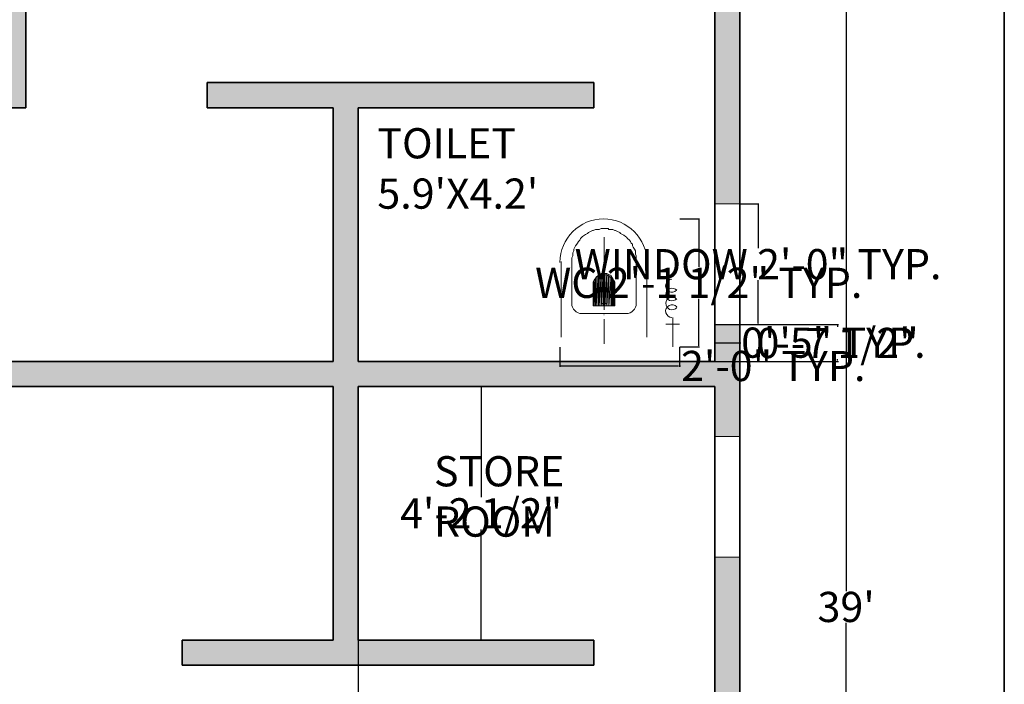
# Model space of a CAD drawing. Units: inches. Extents: x 717 to 1167, y 2046 to 2594.
# Tile 5 of 6: x 972 to 1167, y 2298 to 2430. Entities that reach past the tile are written whole.
import ezdxf

# ---------------------------------------------------------------- set-up
doc = ezdxf.new("R2010")
doc.units = ezdxf.units.IN
doc.header["$MEASUREMENT"] = 0
for name, color, linetype, lineweight in [('A-ANNO-DIMS', 2, 'Continuous', 18), ('A-ANNO-TTLB', 7, 'Continuous', 35), ('A-AREA-IDEN', 7, 'Continuous', 18), ('A-FLOR-FIXT', 8, 'Continuous', 18), ('A-GLAZ', 4, 'Continuous', 18), ('A-WALL', 7, 'Continuous', 35), ('A-WALL-PATT', 140, 'Continuous', 13)]:
    doc.layers.add(name, color=color, linetype=linetype, lineweight=lineweight)
doc.styles.get("Standard").update_dxf_attribs({"font": 'arial.ttf'})
doc.dimstyles.get("Standard").update_dxf_attribs({"dimtxt": 6, "dimasz": 0.18, "dimexe": 0.18, "dimexo": 0.0625, "dimgap": 0.09, "dimtad": 0, "dimtih": 1, "dimtoh": 1, "dimdec": 1, "dimzin": 0, "dimdsep": 46, "dimlunit": 3, "dimtxsty": 'Standard', "dimcen": 0.09, "dimadec": 0, "dimazin": 0, "dimtfac": 1, "dimtdec": 1, "dimtofl": 0, "dimtmove": 0, "dimatfit": 3, "dimfxl": 1, "dimtolj": 1, "dimtzin": 0, "dimarcsym": 0})

# ---------------------------------------------------------------- blocks, each defined once
blk = doc.blocks.new('*D5')
at = {"layer": 'A-ANNO-DIMS', "color": 0, "lineweight": -2, "transparency": 16777216}
for p, q in [((1114.78, 2547.57), (1135.98, 2547.57)), ((1135.8, 2547.39), (1135.8, 2316.73)), ((1135.8, 2079.75), (1135.8, 2310.41)), ((1114.78, 2079.57), (1135.98, 2079.57))]:
    blk.add_line(p, q, dxfattribs=at)
at = {"layer": 'A-ANNO-DIMS', "color": 0, "transparency": 16777216}
for points in [[(1135.77, 2547.39), (1135.83, 2547.39), (1135.8, 2547.57)], [(1135.77, 2079.75), (1135.83, 2079.75), (1135.8, 2079.57)]]:
    blk.add_solid(points, dxfattribs=at)
at = {"layer": 'Defpoints', "color": 0, "transparency": 16777216}
for p in [(1114.71, 2547.57), (1114.71, 2079.57), (1135.8, 2079.57)]:
    blk.add_point(p, dxfattribs=at)
at = {"layer": 'A-ANNO-DIMS', "color": 0, "transparency": 16777216, "insert": (1135.8, 2313.57), "char_height": 6, "attachment_point": 5}
blk.add_mtext("\\A1;39'", dxfattribs=at)
blk = doc.blocks.new('WC-PLAN')
h = blk.add_hatch(color=256)
h.paths.add_polyline_path([(7.21, 8.12), (7.21, 13.81), (7.05, 8.12)])
h.paths.add_polyline_path([(7.21, 13.81), (7.05, 8.12), (7.05, 13.58)])
h = blk.add_hatch(color=256)
h.paths.add_polyline_path([(7.59, 8.12), (7.59, 14.19), (7.21, 8.12)])
h.paths.add_polyline_path([(7.59, 14.19), (7.21, 8.12), (7.21, 13.81)])
h = blk.add_hatch(color=256)
h.paths.add_polyline_path([(7.81, 8.12), (7.81, 14.34), (7.59, 8.12)])
h.paths.add_polyline_path([(7.81, 14.34), (7.59, 8.12), (7.59, 14.19)])
h = blk.add_hatch(color=256)
h.paths.add_polyline_path([(8.19, 8.12), (8.19, 14.56), (7.81, 8.12)])
h.paths.add_polyline_path([(8.19, 14.56), (7.81, 8.12), (7.81, 14.34)])
h = blk.add_hatch(color=256)
h.paths.add_polyline_path([(8.57, 8.12), (8.57, 14.56), (8.19, 8.12)])
h.paths.add_polyline_path([(8.57, 14.56), (8.19, 8.12), (8.19, 14.56)])
h = blk.add_hatch(color=256)
h.paths.add_polyline_path([(8.95, 8.12), (8.95, 14.56), (8.57, 8.12)])
h.paths.add_polyline_path([(8.95, 14.56), (8.57, 8.12), (8.57, 14.56)])
h = blk.add_hatch(color=256)
h.paths.add_polyline_path([(9.33, 8.12), (9.33, 14.56), (8.95, 8.12)])
h.paths.add_polyline_path([(9.33, 14.56), (8.95, 8.12), (8.95, 14.56)])
h = blk.add_hatch(color=256)
h.paths.add_polyline_path([(9.71, 8.12), (9.71, 14.34), (9.33, 8.12)])
h.paths.add_polyline_path([(9.71, 14.34), (9.33, 8.12), (9.33, 14.56)])
h = blk.add_hatch(color=256)
h.paths.add_polyline_path([(10.16, 8.12), (10.16, 14.19), (9.71, 8.12)])
h.paths.add_polyline_path([(10.16, 14.19), (9.71, 8.12), (9.71, 14.34)])
h = blk.add_hatch(color=256)
h.paths.add_polyline_path([(10.32, 8.12), (10.32, 13.81), (10.16, 8.12)])
h.paths.add_polyline_path([(10.32, 13.81), (10.16, 8.12), (10.16, 14.19)])
h = blk.add_hatch(color=256)
h.paths.add_polyline_path([(10.54, 8.12), (10.54, 13.58), (10.32, 8.12)])
h.paths.add_polyline_path([(10.54, 13.58), (10.32, 8.12), (10.32, 13.81)])
h = blk.add_hatch(color=256)
h.paths.add_polyline_path([(6.83, 8.12), (6.83, 13.2), (6.6, 8.12)])
h.paths.add_polyline_path([(6.83, 13.2), (6.6, 8.12), (6.6, 12.82)])
h.paths.add_polyline_path([(6.6, 8.12), (6.6, 12.82), (6.6, 12.44)])
h = blk.add_hatch(color=256)
h.paths.add_polyline_path([(7.05, 8.12), (7.05, 13.58), (6.83, 8.12)])
h.paths.add_polyline_path([(7.05, 13.58), (6.83, 8.12), (6.83, 13.2)])
h = blk.add_hatch(color=256)
h.paths.add_polyline_path([(10.7, 8.12), (10.7, 13.2), (10.54, 8.12)])
h.paths.add_polyline_path([(10.7, 13.2), (10.54, 8.12), (10.54, 13.58)])
h = blk.add_hatch(color=256)
h.paths.add_polyline_path([(10.92, 8.12), (10.92, 12.82), (10.7, 8.12)])
h.paths.add_polyline_path([(10.92, 12.82), (10.7, 8.12), (10.7, 13.2)])
for points in [[(2.35, 15.93), (2.35, 16.69), (2.35, 17.3), (2.35, 17.67), (2.58, 18.05), (2.58, 18.43), (2.58, 18.66), (2.73, 19.04), (2.73, 19.42), (2.96, 19.8), (3.11, 20.03), (3.34, 20.41), (3.49, 20.56), (3.72, 20.94), (3.94, 21.16), (4.1, 21.54), (4.32, 21.77), (4.48, 21.92), (4.85, 22.15), (5.08, 22.3), (5.46, 22.53), (5.69, 22.68), (6.07, 22.91), (6.45, 23.14), (6.6, 23.14), (7.05, 23.29), (7.43, 23.29), (7.81, 23.29), (8.19, 23.52), (8.8, 23.52), (9.56, 23.52), (9.71, 23.29), (10.16, 23.29), (10.54, 23.29), (10.92, 23.14), (11.07, 23.14), (11.45, 22.91), (11.91, 22.68), (12.06, 22.53), (12.44, 22.3), (12.67, 22.15), (13.05, 21.92), (13.2, 21.77), (13.43, 21.54), (13.81, 21.16), (14.03, 20.94), (14.18, 20.56), (14.41, 20.41), (14.41, 20.03), (14.56, 19.8), (14.79, 19.42), (15.02, 19.04), (15.02, 18.66), (15.02, 18.43), (15.17, 18.05), (15.17, 17.67), (15.17, 17.3), (15.17, 16.69), (15.17, 15.93)], [(8.8, 16.92), (8.8, 21.77), (8.8, 21.77)], [(0.23, 1.9), (0.23, 16.92), (0.23, 16.92)], [(2.35, 8.72), (2.35, 15.93), (2.35, 15.93)], [(15.17, 8.72), (15.17, 15.93), (15.17, 15.93)], [(17.29, 1.9), (17.29, 16.92), (17.29, 16.92)], [(8.8, 7.36), (8.8, 14.94), (8.8, 14.94)], [(6.6, 8.12), (6.6, 12.44), (6.6, 12.44)], [(10.92, 8.12), (10.92, 12.44), (10.92, 12.44)], [(6.6, 8.12), (10.92, 8.12), (10.92, 8.12)], [(8.34, 8.57), (8.57, 8.57), (8.8, 8.57)], [(8.34, 8.57), (8.34, 8.5), (8.34, 8.5)], [(8.8, 8.57), (8.72, 8.5), (8.72, 8.5)], [(8.8, 8.57), (8.95, 8.57), (9.18, 8.57)], [(9.18, 8.57), (9.18, 8.5), (9.18, 8.5)], [(4.48, 6.6), (13.2, 6.6), (13.2, 6.6)], [(8.8, 6.37), (8.72, 6.37), (8.72, 6.37)], [(8.8, 0.61), (8.8, 5.46), (8.8, 5.46)], [(21.03, 4.48), (23.77, 4.48), (23.77, 4.48)], [(22.4, 0), (22.4, 5.84), (22.4, 5.84)]]:
    blk.add_lwpolyline(points)
for points in [[(7.21, 8.12), (7.21, 13.81), (7.05, 8.12)], [(7.21, 13.81), (7.05, 8.12), (7.05, 13.58)], [(7.59, 8.12), (7.59, 14.19), (7.21, 8.12)], [(7.59, 14.19), (7.21, 8.12), (7.21, 13.81)], [(7.81, 8.12), (7.81, 14.34), (7.59, 8.12)], [(7.81, 14.34), (7.59, 8.12), (7.59, 14.19)], [(8.19, 8.12), (8.19, 14.56), (7.81, 8.12)], [(8.19, 14.56), (7.81, 8.12), (7.81, 14.34)], [(8.57, 8.12), (8.57, 14.56), (8.19, 8.12)], [(8.57, 14.56), (8.19, 8.12), (8.19, 14.56)], [(8.95, 8.12), (8.95, 14.56), (8.57, 8.12)], [(8.95, 14.56), (8.57, 8.12), (8.57, 14.56)], [(9.33, 8.12), (9.33, 14.56), (8.95, 8.12)], [(9.33, 14.56), (8.95, 8.12), (8.95, 14.56)], [(9.71, 14.34), (9.33, 8.12), (9.33, 14.56)], [(9.71, 8.12), (9.71, 14.34), (9.33, 8.12)], [(10.16, 14.19), (9.71, 8.12), (9.71, 14.34)], [(10.16, 8.12), (10.16, 14.19), (9.71, 8.12)], [(10.32, 13.81), (10.16, 8.12), (10.16, 14.19)], [(10.32, 8.12), (10.32, 13.81), (10.16, 8.12)], [(10.54, 13.58), (10.32, 8.12), (10.32, 13.81)], [(6.83, 8.12), (6.83, 13.2), (6.6, 8.12)], [(6.83, 13.2), (6.6, 8.12), (6.6, 12.82)], [(6.6, 8.12), (6.6, 12.82), (6.6, 12.44)], [(6.6, 12.82), (6.6, 8.12), (6.6, 8.12)], [(7.05, 8.12), (7.05, 13.58), (6.83, 8.12)], [(7.05, 13.58), (6.83, 8.12), (6.83, 13.2)], [(10.54, 8.12), (10.54, 13.58), (10.32, 8.12)], [(10.7, 13.2), (10.54, 8.12), (10.54, 13.58)], [(10.7, 8.12), (10.7, 13.2), (10.54, 8.12)], [(10.92, 12.82), (10.7, 8.12), (10.7, 13.2)], [(10.92, 8.12), (10.92, 12.82), (10.7, 8.12)], [(10.92, 12.44), (10.92, 8.12), (10.92, 12.82)], [(10.92, 8.12), (10.92, 12.44)]]:
    blk.add_lwpolyline(points, close=True)
for points, knots in [([(17.29, 16.76), (17.29, 21.54), (13.43, 25.41), (8.65, 25.41), (8.65, 25.41), (3.87, 25.41), (0, 21.54), (0, 16.76)], [0, 0, 0, 0, 0.125, 0.125, 0.125, 0.125001, 1, 1, 1, 1]), ([(10.7, 12.29), (10.7, 13.43), (9.79, 14.34), (8.65, 14.34), (8.65, 14.34), (7.51, 14.34), (6.6, 13.43), (6.6, 12.29)], [0, 0, 0, 0, 0.125, 0.125, 0.125, 0.125001, 1, 1, 1, 1]), ([(22.25, 13.43), (21.72, 13.43), (21.19, 12.97), (21.03, 12.44), (21.03, 12.44), (20.88, 11.91), (21.19, 11.3), (21.64, 11), (21.64, 11), (22.17, 10.77), (22.78, 10.85), (23.16, 11.23)], [0, 0, 0, 0, 0.083333, 0.083333, 0.083333, 0.083334, 0.166667, 0.166667, 0.166667, 0.166668, 1, 1, 1, 1]), ([(23.23, 11.23), (22.86, 11.61), (22.32, 11.76), (21.79, 11.53), (21.79, 11.53), (21.34, 11.38), (21.03, 10.92), (21.03, 10.39), (21.03, 10.39), (21.03, 9.86), (21.34, 9.41), (21.79, 9.18), (21.79, 9.18), (22.32, 9.03), (22.86, 9.18), (23.23, 9.56)], [0, 0, 0, 0, 0.0625, 0.0625, 0.0625, 0.062501, 0.125, 0.125, 0.125, 0.125001, 0.1875, 0.1875, 0.1875, 0.187501, 1, 1, 1, 1]), ([(23.16, 9.48), (22.86, 9.86), (22.25, 10.01), (21.79, 9.79), (21.79, 9.79), (21.34, 9.63), (21.03, 9.1), (21.03, 8.65), (21.03, 8.65), (21.03, 8.12), (21.34, 7.66), (21.79, 7.43), (21.79, 7.43), (22.32, 7.28), (22.86, 7.43), (23.23, 7.81)], [0, 0, 0, 0, 0.0625, 0.0625, 0.0625, 0.062501, 0.125, 0.125, 0.125, 0.125001, 0.1875, 0.1875, 0.1875, 0.187501, 1, 1, 1, 1]), ([(23.23, 7.96), (22.86, 8.34), (22.17, 8.5), (21.72, 8.19), (21.72, 8.19), (21.19, 7.89), (20.88, 7.36), (21.03, 6.75), (21.03, 6.75), (21.19, 6.22), (21.72, 5.84), (22.25, 5.84)], [0, 0, 0, 0, 0.083333, 0.083333, 0.083333, 0.083334, 0.166667, 0.166667, 0.166667, 0.166668, 1, 1, 1, 1])]:
    blk.add_open_spline(points, degree=3, knots=knots)
for points in [[(2.35, 8.65), (2.35, 7.51), (3.26, 6.6), (4.4, 6.6)], [(13.12, 6.6), (14.26, 6.6), (15.17, 7.51), (15.17, 8.65)]]:
    blk.add_open_spline(points, degree=3)
blk = doc.blocks.new('WINDOW-24IN')
for p, q in [((0, 24), (5, 24)), ((0, 0), (0, 24)), ((5, 24), (5, 0)), ((5, 0), (0, 0))]:
    blk.add_line(p, q)
blk = doc.blocks.new('*D15')
at = {"layer": 'A-ANNO-DIMS', "color": 0, "lineweight": -2, "transparency": 16777216}
for p, q in [((1114.78, 2393.68), (1118.49, 2393.68)), ((1118.31, 2393.5), (1118.31, 2384.87)), ((1118.31, 2369.86), (1118.31, 2378.48)), ((1114.78, 2369.68), (1118.49, 2369.68))]:
    blk.add_line(p, q, dxfattribs=at)
at = {"layer": 'A-ANNO-DIMS', "color": 0, "transparency": 16777216}
for points in [[(1118.28, 2393.5), (1118.34, 2393.5), (1118.31, 2393.68)], [(1118.28, 2369.86), (1118.34, 2369.86), (1118.31, 2369.68)]]:
    blk.add_solid(points, dxfattribs=at)
at = {"layer": 'Defpoints', "color": 0, "transparency": 16777216}
for p in [(1114.71, 2393.68), (1118.31, 2393.68), (1114.71, 2369.68)]:
    blk.add_point(p, dxfattribs=at)
at = {"layer": 'A-ANNO-DIMS', "color": 0, "transparency": 16777216, "insert": (1118.31, 2381.68), "char_height": 6, "attachment_point": 5}
blk.add_mtext('\\A1;WINDOW 2\'-0" TYP.', dxfattribs=at)
blk = doc.blocks.new('*D16')
at = {"layer": 'A-ANNO-DIMS', "color": 0, "lineweight": -2, "transparency": 16777216}
for p, q in [((1109.71, 2369.61), (1109.71, 2365.9)), ((1114.71, 2369.61), (1114.71, 2365.9)), ((1109.89, 2366.08), (1114.53, 2366.08)), ((1114.71, 2366.08), (1114.89, 2366.08))]:
    blk.add_line(p, q, dxfattribs=at)
at = {"layer": 'A-ANNO-DIMS', "color": 0, "transparency": 16777216}
for points in [[(1109.89, 2366.11), (1109.89, 2366.05), (1109.71, 2366.08)], [(1114.53, 2366.11), (1114.53, 2366.05), (1114.71, 2366.08)]]:
    blk.add_solid(points, dxfattribs=at)
at = {"layer": 'Defpoints', "color": 0, "transparency": 16777216}
for p in [(1109.71, 2369.68), (1114.71, 2369.68), (1114.71, 2366.08)]:
    blk.add_point(p, dxfattribs=at)
at = {"layer": 'A-ANNO-DIMS', "color": 0, "transparency": 16777216, "insert": (1133.27, 2366.08), "char_height": 6, "attachment_point": 5}
blk.add_mtext('\\A1;0\'-5" TYP.', dxfattribs=at)
blk = doc.blocks.new('*D21')
at = {"layer": 'A-ANNO-DIMS', "color": 0, "lineweight": -2, "transparency": 16777216}
for p, q in [((1102.79, 2390.68), (1106.71, 2390.68)), ((1106.53, 2390.5), (1106.53, 2381.16)), ((1106.53, 2365.44), (1106.53, 2374.78)), ((1102.79, 2365.26), (1106.71, 2365.26))]:
    blk.add_line(p, q, dxfattribs=at)
at = {"layer": 'A-ANNO-DIMS', "color": 0, "transparency": 16777216}
for points in [[(1106.5, 2390.5), (1106.56, 2390.5), (1106.53, 2390.68)], [(1106.5, 2365.44), (1106.56, 2365.44), (1106.53, 2365.26)]]:
    blk.add_solid(points, dxfattribs=at)
at = {"layer": 'Defpoints', "color": 0, "transparency": 16777216}
for p in [(1102.72, 2390.68), (1106.53, 2390.68), (1102.72, 2365.26)]:
    blk.add_point(p, dxfattribs=at)
at = {"layer": 'A-ANNO-DIMS', "color": 0, "transparency": 16777216, "insert": (1106.53, 2377.97), "char_height": 6, "attachment_point": 5}
blk.add_mtext('\\A1;WC 2\'-1 1/2" TYP.', dxfattribs=at)
blk = doc.blocks.new('*D22')
at = {"layer": 'A-ANNO-DIMS', "color": 0, "lineweight": -2, "transparency": 16777216}
for p, q in [((1078.96, 2365.2), (1078.96, 2361.27)), ((1102.72, 2365.2), (1102.72, 2361.27)), ((1079.14, 2361.45), (1102.54, 2361.45)), ((1102.72, 2361.45), (1102.9, 2361.45))]:
    blk.add_line(p, q, dxfattribs=at)
at = {"layer": 'A-ANNO-DIMS', "color": 0, "transparency": 16777216}
for points in [[(1079.14, 2361.48), (1079.14, 2361.42), (1078.96, 2361.45)], [(1102.54, 2361.48), (1102.54, 2361.42), (1102.72, 2361.45)]]:
    blk.add_solid(points, dxfattribs=at)
at = {"layer": 'Defpoints', "color": 0, "transparency": 16777216}
for p in [(1078.96, 2365.26), (1102.72, 2365.26), (1102.72, 2361.45)]:
    blk.add_point(p, dxfattribs=at)
at = {"layer": 'A-ANNO-DIMS', "color": 0, "transparency": 16777216, "insert": (1121.33, 2361.45), "char_height": 6, "attachment_point": 5}
blk.add_mtext('\\A1;2\'-0" TYP.', dxfattribs=at)
blk = doc.blocks.new('*D36')
at = {"layer": 'A-ANNO-DIMS', "color": 0, "lineweight": -2, "transparency": 16777216}
for p, q in [((1038.91, 2357.31), (1038.91, 2054.99)), ((1109.71, 2357.31), (1109.71, 2054.99)), ((1039.09, 2055.17), (1063.92, 2055.17)), ((1109.53, 2055.17), (1084.71, 2055.17))]:
    blk.add_line(p, q, dxfattribs=at)
at = {"layer": 'A-ANNO-DIMS', "color": 0, "transparency": 16777216}
for points in [[(1039.09, 2055.2), (1039.09, 2055.14), (1038.91, 2055.17)], [(1109.53, 2055.2), (1109.53, 2055.14), (1109.71, 2055.17)]]:
    blk.add_solid(points, dxfattribs=at)
at = {"layer": 'Defpoints', "color": 0, "transparency": 16777216}
for p in [(1038.91, 2357.37), (1109.71, 2357.37), (1109.71, 2055.17)]:
    blk.add_point(p, dxfattribs=at)
at = {"layer": 'A-ANNO-DIMS', "color": 0, "transparency": 16777216, "insert": (1074.31, 2055.17), "char_height": 6, "attachment_point": 5}
blk.add_mtext('\\A1;5\'-11"', dxfattribs=at)
blk = doc.blocks.new('*D37')
at = {"layer": 'A-ANNO-DIMS', "color": 0, "lineweight": -2, "transparency": 16777216}
for p, q in [((1038.98, 2357.37), (1063.49, 2357.37)), ((1063.31, 2357.19), (1063.31, 2335.36)), ((1063.31, 2307.15), (1063.31, 2328.98)), ((1038.98, 2306.97), (1063.49, 2306.97))]:
    blk.add_line(p, q, dxfattribs=at)
at = {"layer": 'A-ANNO-DIMS', "color": 0, "transparency": 16777216}
for points in [[(1063.28, 2357.19), (1063.34, 2357.19), (1063.31, 2357.37)], [(1063.28, 2307.15), (1063.34, 2307.15), (1063.31, 2306.97)]]:
    blk.add_solid(points, dxfattribs=at)
at = {"layer": 'Defpoints', "color": 0, "transparency": 16777216}
for p in [(1038.91, 2357.37), (1038.91, 2306.97), (1063.31, 2306.97)]:
    blk.add_point(p, dxfattribs=at)
at = {"layer": 'A-ANNO-DIMS', "color": 0, "transparency": 16777216, "insert": (1063.31, 2332.17), "char_height": 6, "attachment_point": 5}
blk.add_mtext('\\A1;4\'-2 1/2"', dxfattribs=at)
blk = doc.blocks.new('*D45')
at = {"layer": 'A-ANNO-DIMS', "color": 0, "lineweight": -2, "transparency": 16777216}
for p, q in [((1109.78, 2369.68), (1134.29, 2369.68)), ((1134.11, 2369.5), (1134.11, 2369.22)), ((1109.78, 2362.37), (1134.29, 2362.37)), ((1134.11, 2362.55), (1134.11, 2362.83))]:
    blk.add_line(p, q, dxfattribs=at)
at = {"layer": 'A-ANNO-DIMS', "color": 0, "transparency": 16777216}
for points in [[(1134.08, 2369.5), (1134.14, 2369.5), (1134.11, 2369.68)], [(1134.08, 2362.55), (1134.14, 2362.55), (1134.11, 2362.37)]]:
    blk.add_solid(points, dxfattribs=at)
at = {"layer": 'Defpoints', "color": 0, "transparency": 16777216}
for p in [(1109.71, 2369.68), (1109.71, 2362.37), (1134.11, 2362.37)]:
    blk.add_point(p, dxfattribs=at)
at = {"layer": 'A-ANNO-DIMS', "color": 0, "transparency": 16777216, "insert": (1134.11, 2366.02), "char_height": 6, "attachment_point": 5}
blk.add_mtext('\\A1;0\'-7 1/2"', dxfattribs=at)

msp = doc.modelspace()

# ---------------------------------------------------------------- hatches: boundary and pattern name
at = {"layer": 'A-WALL-PATT'}
h = msp.add_hatch(color=256, dxfattribs=at)
h.dxf.hatch_style = 1
h.paths.add_polyline_path([(796.2, 2547.57), (754.71, 2547.57), (754.71, 2325.38), (759.71, 2325.38), (759.71, 2357.37), (840.31, 2357.37), (840.31, 2362.37), (759.71, 2362.37), (759.71, 2412.77), (835.31, 2412.77), (835.31, 2386.37), (840.31, 2386.37), (840.31, 2412.77), (901.51, 2412.77), (901.51, 2417.77), (759.71, 2417.77), (759.71, 2542.57), (796.2, 2542.57)])
h.paths.add_polyline_path([(913.34, 2547.57), (856.2, 2547.57), (856.2, 2542.57), (896.51, 2542.57), (896.51, 2453.77), (901.51, 2453.77), (901.51, 2542.57), (913.34, 2542.57)])
h.paths.add_polyline_path([(1012.57, 2547.57), (949.34, 2547.57), (949.34, 2542.57), (967.91, 2542.57), (967.91, 2412.77), (972.91, 2412.77), (972.91, 2542.57), (1012.57, 2542.57)])
h.paths.add_polyline_path([(1114.71, 2547.57), (1072.57, 2547.57), (1072.57, 2542.57), (1109.71, 2542.57), (1109.71, 2517.4), (1114.71, 2517.4)])
h.paths.add_polyline_path([(1114.71, 2457.4), (1109.71, 2457.4), (1109.71, 2393.68), (1114.71, 2393.68)])
h.paths.add_polyline_path([(1114.71, 2369.68), (1109.71, 2369.68), (1109.71, 2362.37), (1038.91, 2362.37), (1038.91, 2412.77), (1085.71, 2412.77), (1085.71, 2417.77), (1008.91, 2417.77), (1008.91, 2412.77), (1033.91, 2412.77), (1033.91, 2362.37), (916.31, 2362.37), (916.31, 2357.37), (1033.91, 2357.37), (1033.91, 2306.97), (1003.91, 2306.97), (1003.91, 2301.97), (1085.71, 2301.97), (1085.71, 2306.97), (1038.91, 2306.97), (1038.91, 2357.37), (1109.71, 2357.37), (1109.71, 2347.44), (1114.71, 2347.44)])
h.paths.add_polyline_path([(788.58, 2239.77), (759.71, 2239.77), (759.71, 2265.38), (754.71, 2265.38), (754.71, 2234.77), (788.58, 2234.77)])
h.paths.add_polyline_path([(880.31, 2362.37), (875.31, 2362.37), (875.31, 2239.77), (848.58, 2239.77), (848.58, 2234.77), (875.31, 2234.77), (875.31, 2079.57), (880.31, 2079.57)])
h.paths.add_polyline_path([(1008.91, 2265.97), (1003.91, 2265.97), (1003.91, 2127.77), (991.51, 2127.77), (991.51, 2122.77), (1003.91, 2122.77), (1003.91, 2079.57), (1036.96, 2079.57), (1036.96, 2084.57), (1008.91, 2084.57)])
h.paths.add_polyline_path([(931.51, 2127.77), (916.31, 2127.77), (916.31, 2122.77), (931.51, 2122.77)])
h.paths.add_polyline_path([(1114.71, 2162.57), (1109.71, 2162.57), (1109.71, 2084.57), (1096.96, 2084.57), (1096.96, 2079.57), (1114.71, 2079.57)])
h.paths.add_polyline_path([(1114.71, 2211.37), (1109.71, 2211.37), (1109.71, 2191.57), (1044.91, 2191.57), (1044.91, 2186.57), (1114.71, 2186.57)])
h.paths.add_polyline_path([(1114.71, 2323.44), (1109.71, 2323.44), (1109.71, 2271.37), (1114.71, 2271.37)])

# ---------------------------------------------------------------- linework, layer by layer
at = {"layer": 'A-ANNO-TTLB'}
msp.add_lwpolyline([(719.86, 2594.22), (1167.21, 2594.22), (1167.21, 2050.08), (719.86, 2050.08)], close=True, dxfattribs=at)
at = {"layer": 'A-WALL'}
for p, q in [((1114.71, 2547.57), (1114.71, 2079.57)), ((972.91, 2542.57), (972.91, 2412.77)), ((1109.71, 2542.57), (1109.71, 2362.37)), ((1008.91, 2417.77), (1008.91, 2412.77)), ((1008.91, 2417.77), (1085.71, 2417.77)), ((1085.71, 2417.77), (1085.71, 2412.77)), ((967.91, 2412.77), (972.91, 2412.77)), ((1008.91, 2412.77), (1033.91, 2412.77)), ((1033.91, 2412.77), (1033.91, 2362.37)), ((1033.91, 2412.77), (1033.91, 2362.37)), ((1038.91, 2412.77), (1038.91, 2362.37)), ((1038.91, 2412.77), (1038.91, 2362.37)), ((1038.91, 2412.77), (1085.71, 2412.77)), ((916.31, 2362.37), (1033.91, 2362.37)), ((1038.91, 2362.37), (1109.71, 2362.37)), ((916.31, 2357.37), (1033.91, 2357.37)), ((1033.91, 2357.37), (1033.91, 2306.97)), ((1038.91, 2357.37), (1038.91, 2306.97)), ((1038.91, 2357.37), (1109.71, 2357.37)), ((1109.71, 2357.37), (1109.71, 2191.57)), ((1003.91, 2306.97), (1003.91, 2301.97)), ((1003.91, 2306.97), (1033.91, 2306.97)), ((1038.91, 2306.97), (1085.71, 2306.97)), ((1085.71, 2306.97), (1085.71, 2301.97)), ((1003.91, 2301.97), (1085.71, 2301.97))]:
    msp.add_line(p, q, dxfattribs=at)

# ---------------------------------------------------------------- block references
at = {"layer": 'A-FLOR-FIXT'}
msp.add_blockref('WC-PLAN', (1078.96, 2365.26), dxfattribs=at)
at = {"layer": 'A-GLAZ'}
for p in [(1109.71, 2369.68), (1109.71, 2323.44)]:
    msp.add_blockref('WINDOW-24IN', p, dxfattribs=at)

# ---------------------------------------------------------------- texts
at = {"layer": 'A-AREA-IDEN', "char_height": 6, "attachment_point": 1}
for s, width, insert in [("TOILET\\P5.9'X4.2'", 38.6053, (1042.7, 2408.7)), ('STORE\\PROOM', 41.3597, (1053.95, 2343.53))]:
    msp.add_mtext_dynamic_manual_height_columns(s, width=width, gutter_width=30, heights=[0], dxfattribs=dict(at, insert=insert))

# ---------------------------------------------------------------- dimensions: what is measured, and where the dimension line sits
at = {"layer": 'A-ANNO-DIMS'}
for base, p1, p2, angle, override, picture, middle in [((1135.8, 2079.57), (1114.71, 2547.57), (1114.71, 2079.57), 90, {"dimclrd": 0, "dimclre": 0, "dimclrt": 0}, '*D5', (1135.8, 2313.57)), ((1134.11, 2362.37), (1109.71, 2369.68), (1109.71, 2362.37), 270, {"dimdec": 1, "dimlfac": 1, "dimrnd": 0, "dimzin": 1, "dimdsep": 46, "dimlunit": 4, "dimfrac": 2}, '*D45', (1134.11, 2366.02)), ((1063.31, 2306.97), (1038.91, 2357.37), (1038.91, 2306.97), 270, {"dimdec": 1, "dimlfac": 1, "dimrnd": 0, "dimzin": 1, "dimdsep": 46, "dimlunit": 4, "dimfrac": 2}, '*D37', (1063.31, 2332.17))]:
    dim = msp.add_linear_dim(base=base, p1=p1, p2=p2, angle=angle, dimstyle='Standard', override=override, dxfattribs=at)
    dim.commit()
    dim.dimension.update_dxf_attribs({"geometry": picture, "text_midpoint": middle})
for base, p1, p2, text, picture, middle in [((1106.53, 2390.68), (1102.72, 2365.26), (1102.72, 2390.68), 'WC <> TYP.', '*D21', (1106.53, 2377.97)), ((1118.31, 2393.68), (1114.71, 2369.68), (1114.71, 2393.68), 'WINDOW <> TYP.', '*D15', (1118.31, 2381.68))]:
    dim = msp.add_linear_dim(base=base, p1=p1, p2=p2, angle=90, text=text, dimstyle='Standard', override={"dimdec": 1, "dimlfac": 1, "dimrnd": 0, "dimzin": 1, "dimdsep": 46, "dimlunit": 4, "dimfrac": 2}, dxfattribs=at)
    dim.commit()
    dim.dimension.update_dxf_attribs({"geometry": picture, "text_midpoint": middle})
for base, p1, p2, picture, middle in [((1114.71, 2366.08), (1109.71, 2369.68), (1114.71, 2369.68), '*D16', (1133.27, 2366.08)), ((1102.72, 2361.45), (1078.96, 2365.26), (1102.72, 2365.26), '*D22', (1121.33, 2361.45))]:
    dim = msp.add_linear_dim(base=base, p1=p1, p2=p2, text='<> TYP.', dimstyle='Standard', override={"dimdec": 1, "dimlfac": 1, "dimrnd": 0, "dimzin": 1, "dimdsep": 46, "dimlunit": 4, "dimfrac": 2}, dxfattribs=at)
    dim.commit()
    dim.dimension.update_dxf_attribs({"geometry": picture, "text_midpoint": middle})
dim = msp.add_linear_dim(base=(1109.71, 2055.17), p1=(1038.91, 2357.37), p2=(1109.71, 2357.37), dimstyle='Standard', override={"dimdec": 1, "dimlfac": 1, "dimrnd": 0, "dimzin": 1, "dimdsep": 46, "dimlunit": 4, "dimfrac": 2}, dxfattribs=at)
dim.commit()
dim.dimension.update_dxf_attribs({"geometry": '*D36', "text_midpoint": (1074.31, 2055.17)})

doc.saveas('drawing.dxf')
